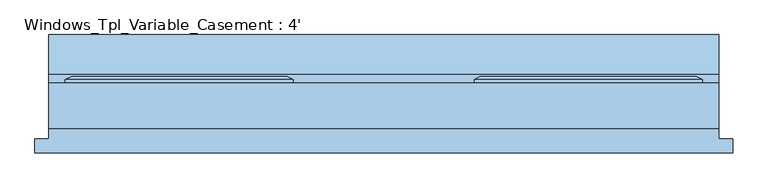
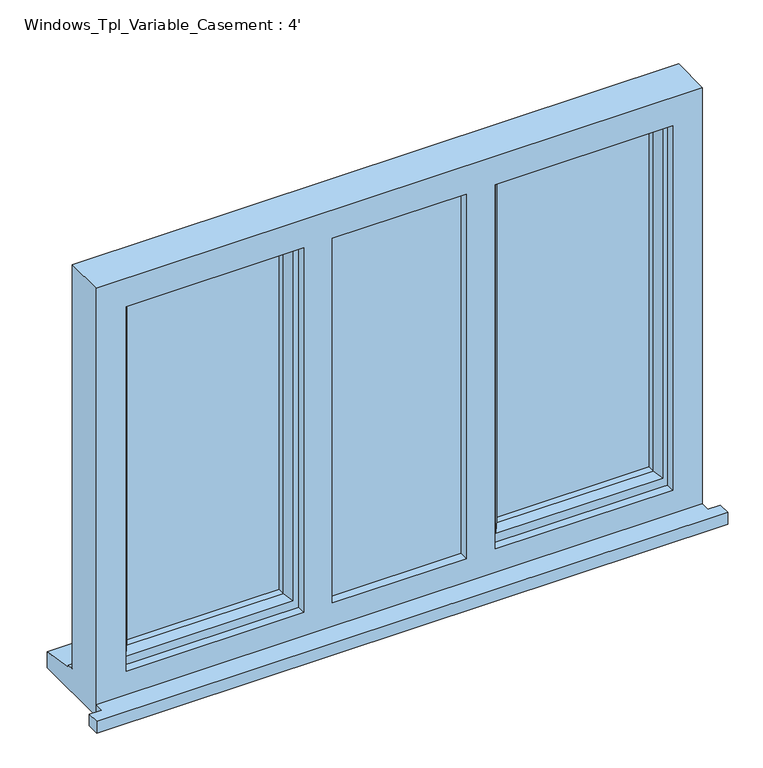
"""IFC4 building model written with IfcOpenShell, lengths in millimetres: window geometry, Windows_Tpl_Variable_Casement : 4'."""

from ifc_helpers import new_model, si_unit, frame, origin, place, context, project, spatial, polyline, outline, extrude, faceted_brep, source, transform, mapped, element, save


def windows_tpl_variable_casement_4_346b9f46(model_context):
    return source(origin(), model_context, "Body", "SolidModel", [
        extrude(outline(polyline([(-929.2, -92.7434322), (-929.2, -67.7434322), (-904.2, -67.7434322), (-904.2, -48.3434322), (315.0, -48.3434322), (315.0, -67.7434322), (340.0, -67.7434322), (340.0, -92.7434322), (-929.2, -92.7434322)])), frame((0.0, 0.0, 1200.0), z_axis=(0.0, 0.0, 1.0), x_axis=(1.0, 0.0, 0.0)), (0.0, 0.0, 1.0), 25.0),
        faceted_brep([(-130.0, 34.6565678, 2080.0), (-130.0, 40.4300705, 2080.0), (-130.0, 40.4300705, 1253.0), (-130.0, 34.6565678, 1253.0), (-120.0, -30.3434322, 2070.0), (-120.0, 34.6565678, 2070.0), (-120.0, 34.6565678, 1263.0), (-120.0, -30.3434322, 1263.0), (-80.0, -15.8505323, 2030.0), (-90.1480377, -30.3434322, 2040.1480377), (-90.1480377, -30.3434322, 1292.8519623), (-80.0, -15.8505323, 1303.0), (-80.0, -1.3434322, 2030.0), (-80.0, -1.3434322, 1303.0), (-90.0, 22.6565678, 2040.0), (-90.0, -1.3434322, 2040.0), (-90.0, -1.3434322, 1293.0), (-90.0, 22.6565678, 1293.0), (-80.0, 40.4300705, 2030.0), (-80.0, 22.6565678, 2030.0), (-80.0, 22.6565678, 1303.0), (-80.0, 40.4300705, 1303.0), (-97.4457548, 46.2035732, 2047.4457548), (-97.4457548, 46.2035732, 1285.5542452), (-119.2153903, 46.2035732, 2069.2153903), (-119.2153903, 46.2035732, 1263.7846097), (285.0, 40.4300705, 1253.0), (285.0, 34.6565678, 1253.0), (275.0, 34.6565678, 1263.0), (275.0, -30.3434322, 1263.0), (245.1480377, -30.3434322, 1292.8519623), (235.0, -15.8505323, 1303.0), (235.0, -1.3434322, 1303.0), (245.0, -1.3434322, 1293.0), (245.0, 22.6565678, 1293.0), (235.0, 22.6565678, 1303.0), (235.0, 40.4300705, 1303.0), (252.4457548, 46.2035732, 1285.5542452), (274.2153903, 46.2035732, 1263.7846097), (285.0, 40.4300705, 2080.0), (285.0, 34.6565678, 2080.0), (275.0, 34.6565678, 2070.0), (275.0, -30.3434322, 2070.0), (245.1480377, -30.3434322, 2040.1480377), (235.0, -15.8505323, 2030.0), (235.0, -1.3434322, 2030.0), (245.0, -1.3434322, 2040.0), (245.0, 22.6565678, 2040.0), (235.0, 22.6565678, 2030.0), (235.0, 40.4300705, 2030.0), (252.4457548, 46.2035732, 2047.4457548), (274.2153903, 46.2035732, 2069.2153903)], [[[0, 1, 2, 3]], [[4, 5, 6, 7]], [[8, 9, 10, 11]], [[12, 8, 11, 13]], [[14, 15, 16, 17]], [[18, 19, 20, 21]], [[22, 18, 21, 23]], [[1, 24, 25, 2]], [[3, 2, 26, 27]], [[7, 6, 28, 29]], [[11, 10, 30, 31]], [[13, 11, 31, 32]], [[17, 16, 33, 34]], [[21, 20, 35, 36]], [[23, 21, 36, 37]], [[2, 25, 38, 26]], [[27, 26, 39, 40]], [[29, 28, 41, 42]], [[31, 30, 43, 44]], [[32, 31, 44, 45]], [[34, 33, 46, 47]], [[36, 35, 48, 49]], [[37, 36, 49, 50]], [[26, 38, 51, 39]], [[40, 39, 1, 0]], [[3, 27, 40, 0], [5, 41, 28, 6]], [[42, 41, 5, 4]], [[7, 29, 42, 4], [9, 43, 30, 10]], [[44, 43, 9, 8]], [[45, 44, 8, 12]], [[15, 46, 33, 16], [13, 32, 45, 12]], [[47, 46, 15, 14]], [[17, 34, 47, 14], [19, 48, 35, 20]], [[49, 48, 19, 18]], [[50, 49, 18, 22]], [[24, 51, 38, 25], [23, 37, 50, 22]], [[39, 51, 24, 1]]]),
        faceted_brep([(-459.2, 34.6565678, 2080.0), (-459.2, 40.4300705, 2080.0), (-874.2, 40.4300705, 2080.0), (-874.2, 34.6565678, 2080.0), (-469.2, -30.3434322, 2070.0), (-469.2, 34.6565678, 2070.0), (-864.2, 34.6565678, 2070.0), (-864.2, -30.3434322, 2070.0), (-509.2, -15.8505323, 2030.0), (-499.0519623, -30.3434322, 2040.1480377), (-834.3480377, -30.3434322, 2040.1480377), (-824.2, -15.8505323, 2030.0), (-509.2, -1.3434322, 2030.0), (-824.2, -1.3434322, 2030.0), (-499.2, 22.6565678, 2040.0), (-499.2, -1.3434322, 2040.0), (-834.2, -1.3434322, 2040.0), (-834.2, 22.6565678, 2040.0), (-509.2, 40.4300705, 2030.0), (-509.2, 22.6565678, 2030.0), (-824.2, 22.6565678, 2030.0), (-824.2, 40.4300705, 2030.0), (-490.3854344, 46.2035732, 2048.8145656), (-843.0145656, 46.2035732, 2048.8145656), (-470.8307806, 46.2035732, 2068.3692194), (-862.5692194, 46.2035732, 2068.3692194), (-874.2, 40.4300705, 1253.0), (-874.2, 34.6565678, 1253.0), (-864.2, 34.6565678, 1263.0), (-864.2, -30.3434322, 1263.0), (-834.3480377, -30.3434322, 1292.8519623), (-824.2, -15.8505323, 1303.0), (-824.2, -1.3434322, 1303.0), (-834.2, -1.3434322, 1293.0), (-834.2, 22.6565678, 1293.0), (-824.2, 22.6565678, 1303.0), (-824.2, 40.4300705, 1303.0), (-843.0145656, 46.2035732, 1284.1854344), (-862.5692194, 46.2035732, 1264.6307806), (-459.2, 40.4300705, 1253.0), (-459.2, 34.6565678, 1253.0), (-469.2, 34.6565678, 1263.0), (-469.2, -30.3434322, 1263.0), (-499.0519623, -30.3434322, 1292.8519623), (-509.2, -15.8505323, 1303.0), (-509.2, -1.3434322, 1303.0), (-499.2, -1.3434322, 1293.0), (-499.2, 22.6565678, 1293.0), (-509.2, 22.6565678, 1303.0), (-509.2, 40.4300705, 1303.0), (-490.3854344, 46.2035732, 1284.1854344), (-470.8307806, 46.2035732, 1264.6307806)], [[[0, 1, 2, 3]], [[4, 5, 6, 7]], [[8, 9, 10, 11]], [[12, 8, 11, 13]], [[14, 15, 16, 17]], [[18, 19, 20, 21]], [[22, 18, 21, 23]], [[1, 24, 25, 2]], [[3, 2, 26, 27]], [[7, 6, 28, 29]], [[11, 10, 30, 31]], [[13, 11, 31, 32]], [[17, 16, 33, 34]], [[21, 20, 35, 36]], [[23, 21, 36, 37]], [[2, 25, 38, 26]], [[27, 26, 39, 40]], [[0, 3, 27, 40], [41, 28, 6, 5]], [[29, 28, 41, 42]], [[4, 7, 29, 42], [43, 30, 10, 9]], [[31, 30, 43, 44]], [[32, 31, 44, 45]], [[46, 33, 16, 15], [12, 13, 32, 45]], [[34, 33, 46, 47]], [[14, 17, 34, 47], [48, 35, 20, 19]], [[36, 35, 48, 49]], [[37, 36, 49, 50]], [[51, 38, 25, 24], [22, 23, 37, 50]], [[26, 38, 51, 39]], [[40, 39, 1, 0]], [[42, 41, 5, 4]], [[44, 43, 9, 8]], [[45, 44, 8, 12]], [[47, 46, 15, 14]], [[49, 48, 19, 18]], [[50, 49, 18, 22]], [[39, 51, 24, 1]]]),
        faceted_brep([(315.0, -48.3434322, 2110.0), (-904.2, -48.3434322, 2110.0), (-904.2, -48.3434322, 1200.0), (315.0, -48.3434322, 1200.0), (255.0, -48.3434322, 2050.0), (255.0, -48.3434322, 1275.0), (-102.0, -48.3434322, 1275.0), (-102.0, -48.3434322, 2050.0), (-487.2, -48.3434322, 2050.0), (-487.2, -48.3434322, 1275.0), (-844.2, -48.3434322, 1275.0), (-844.2, -48.3434322, 2050.0), (-160.0, -48.3434322, 2050.0), (-160.0, -48.3434322, 1275.0), (-429.2, -48.3434322, 1275.0), (-429.2, -48.3434322, 2050.0), (-904.2, 34.6565678, 2110.0), (-904.2, 34.6565678, 1251.0), (-904.2, 49.6565678, 1249.68767), (-904.2, 49.6565678, 1244.7449676), (-904.2, 122.1565678, 1233.8088847), (-904.2, 122.1565678, 1200.0), (315.0, 34.6565678, 2110.0), (315.0, 34.6565678, 1251.0), (-864.2, 34.6565678, 2070.0), (-864.2, 34.6565678, 1263.0), (-469.2, 34.6565678, 1263.0), (-469.2, 34.6565678, 2070.0), (-429.2, 34.6565678, 2070.0), (-429.2, 34.6565678, 1263.0), (-160.0, 34.6565678, 1263.0), (-160.0, 34.6565678, 2070.0), (-120.0, 34.6565678, 2070.0), (-120.0, 34.6565678, 1263.0), (275.0, 34.6565678, 1263.0), (275.0, 34.6565678, 2070.0), (-864.2, -30.3434322, 2070.0), (-864.2, -30.3434322, 1263.0), (-469.2, -30.3434322, 2070.0), (-469.2, -30.3434322, 1263.0), (-487.2, -30.3434322, 2050.0), (-844.2, -30.3434322, 2050.0), (-844.2, -30.3434322, 1275.0), (-487.2, -30.3434322, 1275.0), (-439.2, -30.3434322, 2070.0), (-150.0, -30.3434322, 2070.0), (-150.0, -30.3434322, 1263.0), (-439.2, -30.3434322, 1263.0), (-160.0, -30.3434322, 2050.0), (-429.2, -30.3434322, 2050.0), (-429.2, -30.3434322, 1275.0), (-160.0, -30.3434322, 1275.0), (-120.0, -30.3434322, 2070.0), (275.0, -30.3434322, 2070.0), (275.0, -30.3434322, 1263.0), (-120.0, -30.3434322, 1263.0), (255.0, -30.3434322, 2050.0), (-102.0, -30.3434322, 2050.0), (-102.0, -30.3434322, 1275.0), (255.0, -30.3434322, 1275.0), (-429.2, -6.3434322, 2070.0), (-160.0, -6.3434322, 2070.0), (-150.0, -6.3434322, 2070.0), (-439.2, -6.3434322, 2070.0), (315.0, 122.1565678, 1200.0), (315.0, 122.1565678, 1233.8088847), (315.0, 49.6565678, 1244.7449676), (315.0, 49.6565678, 1249.68767), (-429.2, -6.3434322, 1263.0), (-150.0, -6.3434322, 1263.0), (-160.0, -6.3434322, 1263.0), (-439.2, -6.3434322, 1263.0)], [[[0, 1, 2, 3], [4, 5, 6, 7], [8, 9, 10, 11], [12, 13, 14, 15]], [[2, 1, 16, 17, 18, 19, 20, 21]], [[17, 16, 22, 23], [24, 25, 26, 27], [28, 29, 30, 31], [32, 33, 34, 35]], [[25, 24, 36, 37]], [[36, 38, 39, 37], [40, 41, 42, 43]], [[44, 45, 46, 47], [48, 49, 50, 51]], [[52, 53, 54, 55], [56, 57, 58, 59]], [[41, 11, 10, 42]], [[1, 0, 22, 16]], [[36, 24, 27, 38]], [[35, 53, 52, 32]], [[60, 28, 31, 61, 62, 45, 44, 63]], [[11, 41, 40, 8]], [[56, 4, 7, 57]], [[15, 49, 48, 12]], [[23, 22, 0, 3, 64, 65, 66, 67]], [[35, 34, 54, 53]], [[4, 56, 59, 5]], [[8, 40, 43, 9]], [[27, 26, 39, 38]], [[29, 28, 60, 68]], [[57, 7, 6, 58]], [[64, 3, 2, 21]], [[65, 64, 21, 20]], [[66, 65, 20, 19]], [[67, 66, 19, 18]], [[23, 67, 18, 17]], [[34, 33, 55, 54]], [[26, 25, 37, 39]], [[47, 46, 69, 70, 30, 29, 68, 71]], [[6, 5, 59, 58]], [[51, 50, 14, 13]], [[43, 42, 10, 9]], [[49, 15, 14, 50]], [[68, 60, 63, 71]], [[71, 63, 44, 47]], [[62, 69, 46, 45]], [[69, 62, 61, 70]], [[70, 61, 31, 30]], [[33, 32, 52, 55]], [[12, 48, 51, 13]]]),
        extrude(outline(polyline([(-499.2, -1.3434322), (-834.2, -1.3434322), (-834.2, 22.6565678), (-499.2, 22.6565678), (-499.2, -1.3434322)])), frame((0.0, 0.0, 1293.0), z_axis=(0.0, 0.0, 1.0), x_axis=(1.0, 0.0, 0.0)), (0.0, 0.0, 1.0), 747.0),
        extrude(outline(polyline([(-439.2, -6.3434322), (-150.0, -6.3434322), (-150.0, -30.3434322), (-439.2, -30.3434322), (-439.2, -6.3434322)])), frame((0.0, 0.0, 1263.0), z_axis=(0.0, 0.0, 1.0), x_axis=(1.0, 0.0, 0.0)), (0.0, 0.0, 1.0), 807.0),
        extrude(outline(polyline([(245.0, -1.3434322), (-90.0, -1.3434322), (-90.0, 22.6565678), (245.0, 22.6565678), (245.0, -1.3434322)])), frame((0.0, 0.0, 1293.0), z_axis=(0.0, 0.0, 1.0), x_axis=(1.0, 0.0, 0.0)), (0.0, 0.0, 1.0), 747.0),
    ])


if __name__ == "__main__":
    model = new_model("IFC4")
    model_context = context("Model", 3, world=origin())
    ifc_project = project(units=[si_unit("LENGTHUNIT", "METRE", prefix="MILLI")], contexts=[model_context])
    site = spatial("IfcSite", under=ifc_project)
    building = spatial("IfcBuilding", under=site)
    placement = place(None, origin())
    windows_tpl_variable_casement_4_shape = windows_tpl_variable_casement_4_346b9f46(model_context)
    element("IfcWindow", 1, ObjectType="Windows_Tpl_Variable_Casement : 4'", at=placement, inside=building, context=model_context, shape_type="MappedRepresentation", body=[
        mapped(windows_tpl_variable_casement_4_shape, transform((0.0, 0.0, 0.0), x_axis=(1.0, 0.0, 0.0), y_axis=(0.0, 1.0, 0.0), z_axis=(0.0, 0.0, 1.0))),
    ])
    save(model, "model.ifc")

# Revit data of these elements
# Type "Windows_Tpl_Variable_Casement : 4'"
#   Type Mark = "81"
#   Operation = "TriplePanelVertical"
#   Construction Type Id = "GSP4R"
#   Manufacturer = "Revit"
#   Keynote = "L10"
#   Analytic Construction = "1/8 in Pilkington single glazing"
#   Wrap Layers (Int) from Ext = 177.5 mm
#   Wrap Layers (Ext) from Ext = 102.5 mm
#   Window Board Projection = 25 mm
#   Window Board Extension = 25 mm
#   Visual Light Transmittance = 0.9
#   Solar Heat Gain Coefficient = 0.78
#   Rough Width = 1219.2 mm
#   Rough Height = 910 mm
#   Height = 910 mm
#   Width = 1219.2 mm
#   Heat Transfer Coefficient (U) = 3.6886 W/(m²·K)
#   Glazing Thickness = 24 mm
#   FrameOffset - External = 50 mm
#   Frame Depth = 65 mm
#   Default Head Height = 2110 mm
#   Cill Depth = 87.5 mm
#   Cavity Closer Width = 50 mm
#   Cavity Closer Offset from Ext = 102.5 mm
#   Cavity Closer Depth = 85 mm
#   Casement Width = 450 mm
#   Vis - Cavity Closers = yes
#   Define Thermal Properties by = 1
#   Material Trim = Window Frame
#   Material Glass = Glass
#   Material Frame = Window Frame
#   Wall Closure = (empty or 0)
# Element 1 (IfcWindow, "Windows_Tpl_Variable_Casement : 4'")
#   Materials on its faces: "Window Frame", "Glass"
# Materials
#   "Window Frame": colour RGB 249 249 249, transparency 0, Keynote = "L10", Cost = 0
#   "Glass": class "Glass", colour RGB 0 128 192, transparency 0.9, Description = "Soda Lime Glass", Cost = 0
